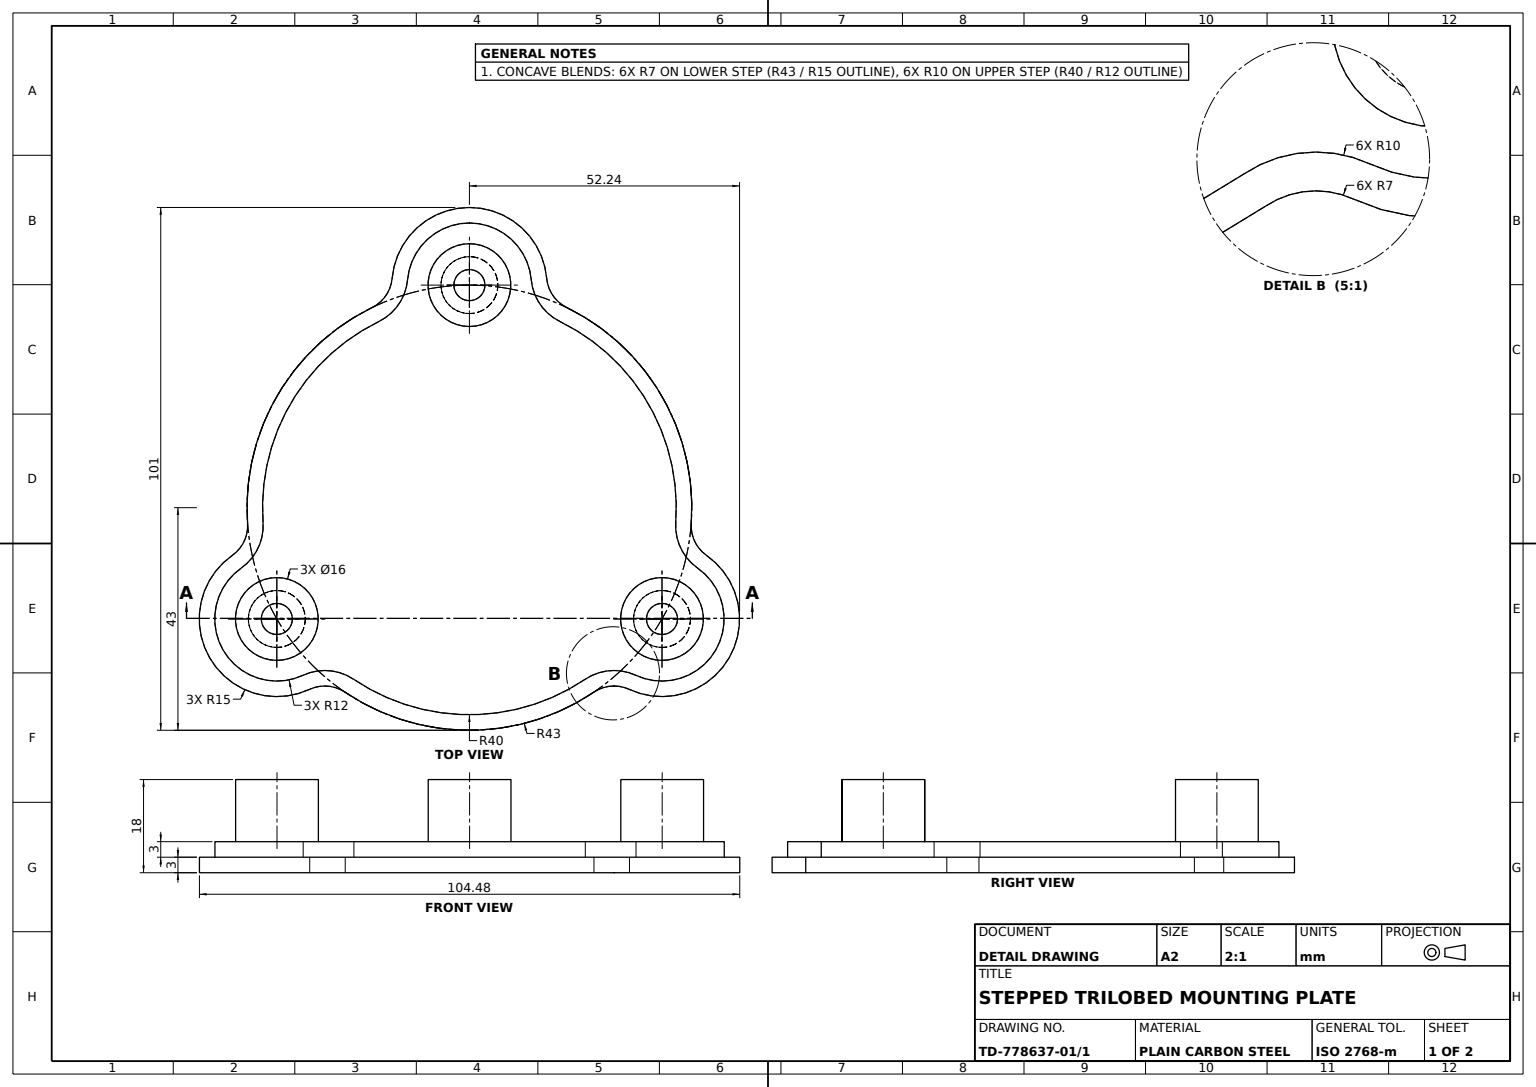
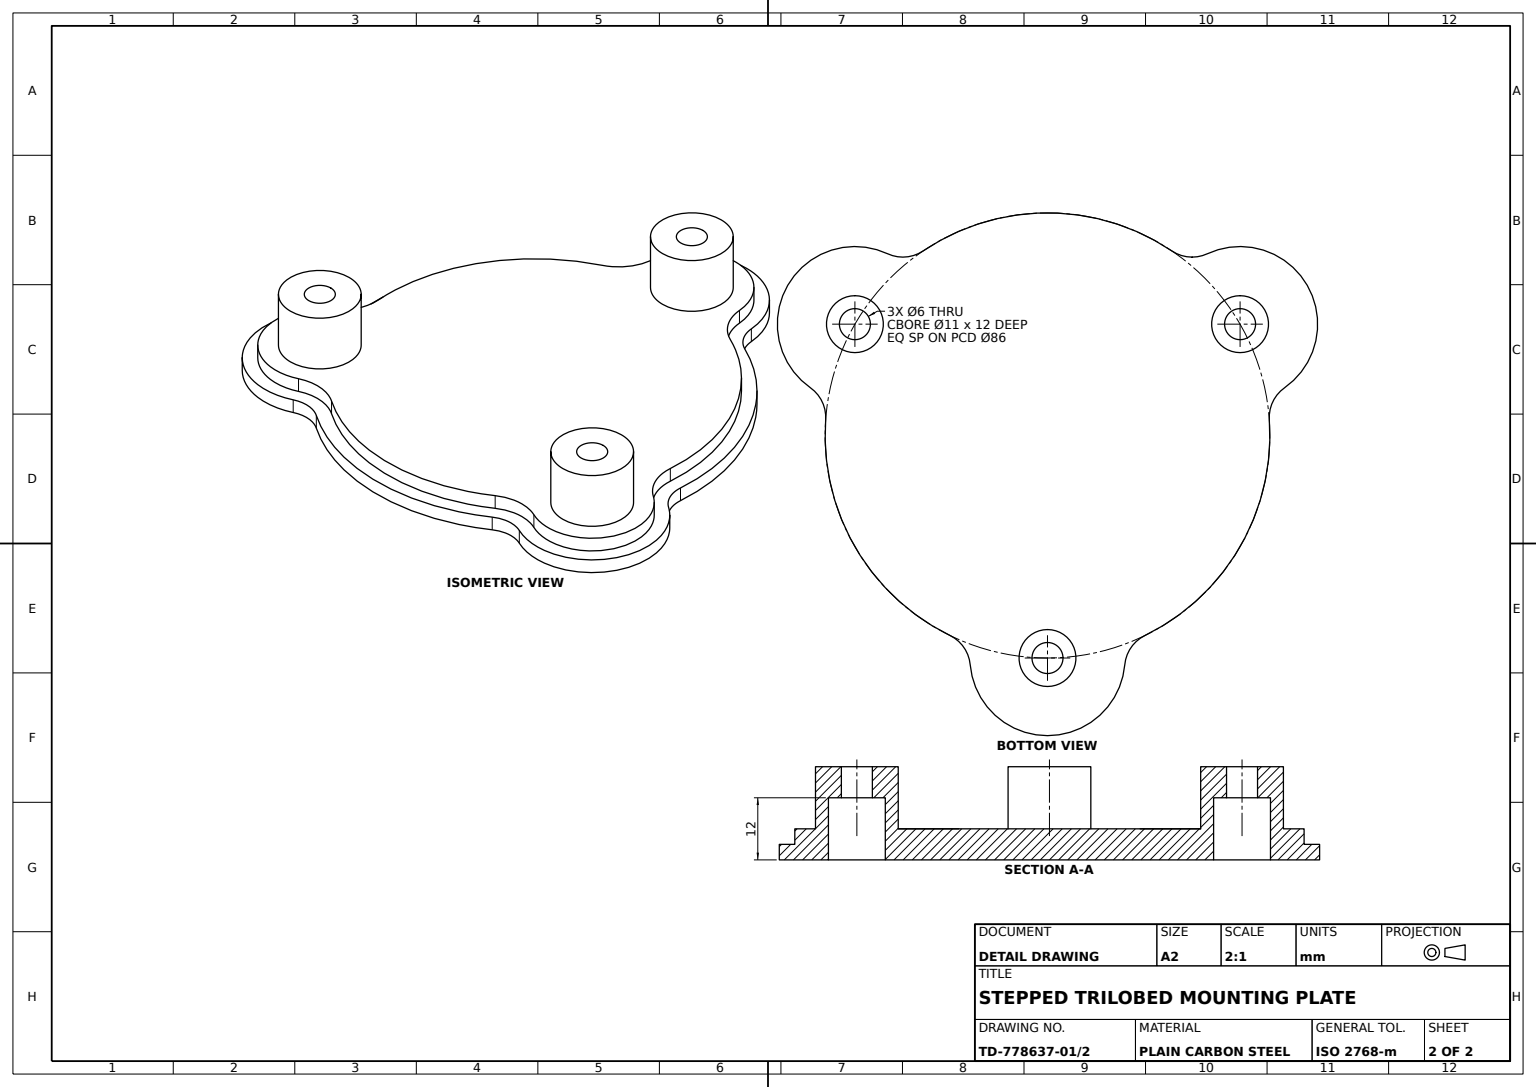
SolidWorks part; units mm, degrees
material "Plain Carbon Steel"
ref_plane "Front Plane" through (0, 0, 0) normal (0, 0, 1) x (1, 0, 0)
ref_plane "Top Plane" through (0, 0, 0) normal (0, 1, 0) x (1, 0, 0)
ref_plane "Right Plane" through (0, 0, 0) normal (1, 0, 0) x (0, 0, -1)
sketch "Base Flange Profile" plane through (0, 0, 0) normal (0, 1, 0) x (1, 0, 0)
  circle A1 centre (0, 43) radius 8
  arc A2 (14.9415, 44.324) -> (-14.9415, 44.324) centre (0, 43) ccw
  arc A3 (30.915, -35.1017) -> (45.8564, -9.2223) centre (37.2391, -21.5) ccw
  circle A4 centre (37.2391, -21.5) radius 8
  arc A5 (-45.8564, -9.2223) -> (-30.915, -35.1017) centre (-37.2391, -21.5) ccw
  circle A6 centre (-37.2391, -21.5) radius 8
  arc A7 (42.895, -3.0038) -> (18.8462, 38.65) centre (0, 0) ccw
  arc A8 (45.8564, -9.2223) -> (42.895, -3.0038) centre (49.8779, -3.4927) cw
  arc A9 (-24.0488, -35.6462) -> (24.0488, -35.6462) centre (0, 0) ccw
  arc A10 (-18.8462, 38.65) -> (-42.895, -3.0038) centre (0, 0) ccw
  arc A11 (30.915, -35.1017) -> (24.0488, -35.6462) centre (27.9637, -41.4491) ccw
  arc A12 (-30.915, -35.1017) -> (-24.0488, -35.6462) centre (-27.9637, -41.4491) cw
  arc A13 (-45.8564, -9.2223) -> (-42.895, -3.0038) centre (-49.8779, -3.4927) ccw
  arc A14 (-14.9415, 44.324) -> (-18.8462, 38.65) centre (-21.9141, 44.9419) cw
  arc A15 (14.9415, 44.324) -> (18.8462, 38.65) centre (21.9141, 44.9419) ccw
  point P14 (0, 0)
  dimension "D1" = 7
  dimension "D2" = 16
  dimension "D3" = 30
  dimension "D5" = 7
  dimension "D6" = 43
  dimension "D7" = 7
  dimension "D4" = 3
extrude "Base Flange 3mm" add sketch "Base Flange Profile" along normal blind 3
sketch "Raised Plate Profile" plane through (0, 3, 0) normal (0, 1, 0) x (1, 0, 0)
  arc A24 (39.9023, -2.7942) -> (44.133, -11.6779) centre (49.8779, -3.4927) ccw
  arc A25 (39.9023, -2.7942) -> (17.5313, 35.9535) centre (0, 0) ccw
  arc A26 (11.9532, 44.0592) -> (17.5313, 35.9535) centre (21.9141, 44.9419) ccw
  arc A27 (11.9532, 44.0592) -> (-11.9532, 44.0592) centre (0, 43) ccw
  arc A28 (-17.5313, 35.9535) -> (-11.9532, 44.0592) centre (-21.9141, 44.9419) ccw
  arc A29 (-17.5313, 35.9535) -> (-39.9023, -2.7942) centre (0, 0) ccw
  arc A30 (-44.133, -11.6779) -> (-39.9023, -2.7942) centre (-49.8779, -3.4927) ccw
  arc A31 (-44.133, -11.6779) -> (-32.1798, -32.3813) centre (-37.2391, -21.5) ccw
  arc A32 (-22.371, -33.1593) -> (-32.1798, -32.3813) centre (-27.9637, -41.4491) ccw
  arc A33 (-22.371, -33.1593) -> (22.371, -33.1593) centre (0, 0) ccw
  arc A34 (32.1798, -32.3813) -> (22.371, -33.1593) centre (27.9637, -41.4491) ccw
  arc A35 (32.1798, -32.3813) -> (44.133, -11.6779) centre (37.2391, -21.5) ccw
  arc A36 (39.9023, -2.7942) -> (44.133, -11.6779) centre (49.8779, -3.4927) ccw
  arc A37 (39.9023, -2.7942) -> (17.5313, 35.9535) centre (0, 0) ccw
  arc A38 (11.9532, 44.0592) -> (17.5313, 35.9535) centre (21.9141, 44.9419) ccw
  arc A39 (11.9532, 44.0592) -> (-11.9532, 44.0592) centre (0, 43) ccw
  arc A40 (-17.5313, 35.9535) -> (-11.9532, 44.0592) centre (-21.9141, 44.9419) ccw
  arc A41 (-17.5313, 35.9535) -> (-39.9023, -2.7942) centre (0, 0) ccw
  arc A42 (-44.133, -11.6779) -> (-39.9023, -2.7942) centre (-49.8779, -3.4927) ccw
  arc A43 (-44.133, -11.6779) -> (-32.1798, -32.3813) centre (-37.2391, -21.5) ccw
  arc A44 (-22.371, -33.1593) -> (-32.1798, -32.3813) centre (-27.9637, -41.4491) ccw
  arc A45 (-22.371, -33.1593) -> (22.371, -33.1593) centre (0, 0) ccw
  arc A46 (32.1798, -32.3813) -> (22.371, -33.1593) centre (27.9637, -41.4491) ccw
  arc A47 (32.1798, -32.3813) -> (44.133, -11.6779) centre (37.2391, -21.5) ccw
  dimension "D1" = 3
extrude "Raised Plate 3mm" add sketch "Raised Plate Profile" along normal blind 3
sketch "Lobe Cut Profile 3x" plane through (0, 0, 0) normal (0, -1, 0) x (1, 0, 0)
  circle A0 centre (0, -43) radius 8 construction
  circle A1 centre (37.2391, 21.5) radius 8 construction
  circle A2 centre (-37.2391, 21.5) radius 8 construction
  circle A3 centre (0, -43) radius 8
  circle A4 centre (37.2391, 21.5) radius 8
  circle A5 centre (-37.2391, 21.5) radius 8
extrude "Lobe Cut 3x 13mm" cut sketch "Lobe Cut Profile 3x" against normal blind 13
sketch "Boss Profile 3x" plane through (0, 6, 0) normal (0, 1, 0) x (1, 0, 0)
  circle A0 centre (0, 43) radius 8 construction
  circle A1 centre (37.2391, -21.5) radius 8 construction
  circle A2 centre (-37.2391, -21.5) radius 8 construction
  circle A3 centre (0, 43) radius 8
  circle A4 centre (37.2391, -21.5) radius 8
  circle A5 centre (-37.2391, -21.5) radius 8
extrude "Bosses 3x" add sketch "Boss Profile 3x" along normal blind 12 and the other way blind 6
sketch "Boss Hole Profile 3x" plane through (0, 0, 0) normal (0, -1, 0) x (1, 0, 0)
  circle A0 centre (0, -43) radius 5.5
  circle A1 centre (37.2391, 21.5) radius 5.5
  circle A2 centre (-37.2391, 21.5) radius 5.5
  circle A3 centre (-37.2391, 21.5) radius 3
  circle A4 centre (0, -43) radius 3
  circle A5 centre (37.2391, 21.5) radius 3
  dimension "D1" = 11
  dimension "D2" = 6
  dimension "D3" = 6
  dimension "D4" = 6
extrude "Boss Holes 3x 12mm" cut sketch "Boss Hole Profile 3x" against normal blind 12
sketch "Through Cut Profile 3x" plane through (0, 0, 0) normal (0, -1, 0) x (1, 0, 0)
  circle A0 centre (0, -43) radius 3 construction
  circle A1 centre (37.2391, 21.5) radius 3 construction
  circle A2 centre (-37.2391, 21.5) radius 3 construction
  circle A3 centre (0, -43) radius 3
  circle A4 centre (37.2391, 21.5) radius 3
  circle A5 centre (-37.2391, 21.5) radius 3
extrude "Through Cut 3x 22mm" cut sketch "Through Cut Profile 3x" against normal blind 22
